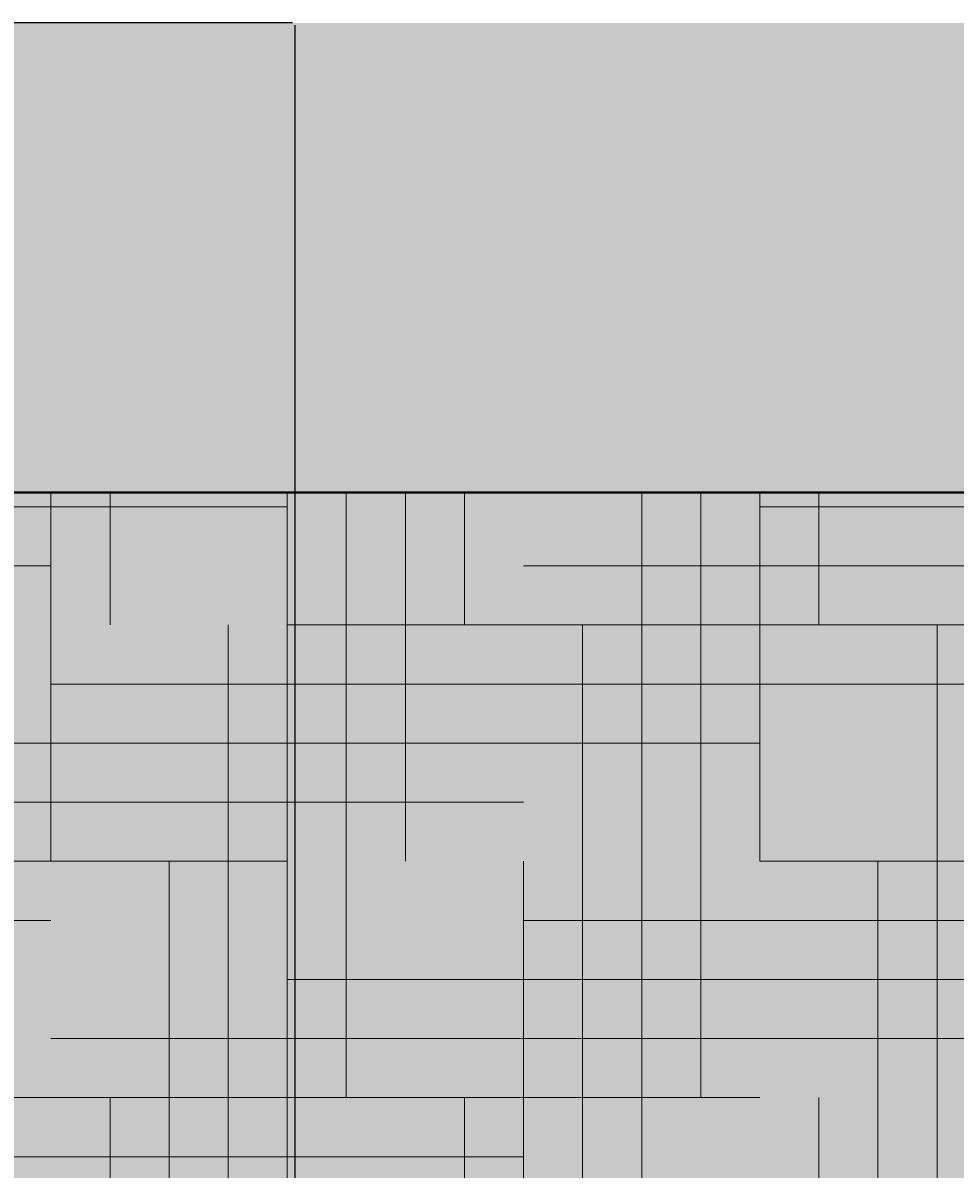
# Model space of a CAD drawing. Units: feet. Extents: x 2695 to 2912, y 795 to 1139.
# Tile 14 of 83: x 2723 to 2748, y 906 to 937. Entities that reach past the tile are written whole.
import ezdxf

# ---------------------------------------------------------------- set-up
doc = ezdxf.new("R2010")
doc.units = ezdxf.units.FT
for name, color, linetype, lineweight in [('A-ANNO-DIMS', 2, 'Continuous', 18), ('A-ELEV', 7, 'Continuous', 35), ('A-ELEV-PATT', 252, 'Continuous', 13)]:
    doc.layers.add(name, color=color, linetype=linetype, lineweight=lineweight)
doc.styles.get("Standard").update_dxf_attribs({"font": 'arial.ttf'})
doc.dimstyles.get("Standard").update_dxf_attribs({"dimtxt": 0.18, "dimasz": 0.18, "dimexe": 0.18, "dimexo": 0.0625, "dimgap": 0.09, "dimtad": 0, "dimtih": 1, "dimtoh": 1, "dimdec": 1, "dimzin": 0, "dimdsep": 46, "dimlunit": 3, "dimtxsty": 'Standard', "dimcen": 0.09, "dimadec": 0, "dimazin": 0, "dimtfac": 1, "dimtdec": 1, "dimtofl": 0, "dimtmove": 0, "dimatfit": 3, "dimfxl": 1, "dimtolj": 1, "dimtzin": 0, "dimarcsym": 0})

# ---------------------------------------------------------------- blocks, each defined once
blk = doc.blocks.new('*D23')
at = {"layer": 'A-ANNO-DIMS', "color": 0, "lineweight": -2, "transparency": 16777216}
for p, q in [((2715.885, 936.868), (2715.885, 794.976)), ((2730.708, 936.868), (2730.708, 794.976)), ((2716.065, 795.156), (2722.842, 795.156)), ((2730.528, 795.156), (2723.752, 795.156))]:
    blk.add_line(p, q, dxfattribs=at)
at = {"layer": 'A-ANNO-DIMS', "color": 0, "transparency": 16777216}
for points in [[(2716.065, 795.186), (2716.065, 795.126), (2715.885, 795.156)], [(2730.528, 795.186), (2730.528, 795.126), (2730.708, 795.156)]]:
    blk.add_solid(points, dxfattribs=at)
at = {"layer": 'Defpoints', "color": 0, "transparency": 16777216}
for p in [(2715.885, 936.931), (2730.708, 936.931), (2730.708, 795.156)]:
    blk.add_point(p, dxfattribs=at)
at = {"layer": 'A-ANNO-DIMS', "color": 0, "transparency": 16777216, "insert": (2723.297, 795.156), "char_height": 0.18, "attachment_point": 5}
blk.add_mtext('\\A1;14.823', dxfattribs=at)
blk = doc.blocks.new('*D24')
at = {"layer": 'A-ANNO-DIMS', "color": 0, "lineweight": -2, "transparency": 16777216}
for p, q in [((2730.708, 936.868), (2730.708, 794.976)), ((2755.112, 936.868), (2755.112, 794.976)), ((2730.888, 795.156), (2742.446, 795.156)), ((2754.932, 795.156), (2743.375, 795.156))]:
    blk.add_line(p, q, dxfattribs=at)
at = {"layer": 'A-ANNO-DIMS', "color": 0, "transparency": 16777216}
for points in [[(2730.888, 795.186), (2730.888, 795.126), (2730.708, 795.156)], [(2754.932, 795.186), (2754.932, 795.126), (2755.112, 795.156)]]:
    blk.add_solid(points, dxfattribs=at)
at = {"layer": 'Defpoints', "color": 0, "transparency": 16777216}
for p in [(2730.708, 936.931), (2755.112, 936.931), (2755.112, 795.156)]:
    blk.add_point(p, dxfattribs=at)
at = {"layer": 'A-ANNO-DIMS', "color": 0, "transparency": 16777216, "insert": (2742.91, 795.156), "char_height": 0.18, "attachment_point": 5}
blk.add_mtext('\\A1;24.404', dxfattribs=at)
blk = doc.blocks.new('*D27')
at = {"layer": 'A-ANNO-DIMS', "color": 0, "lineweight": -2, "transparency": 16777216}
for p, q in [((2730.646, 938.518), (2694.681, 938.518)), ((2694.861, 938.338), (2694.861, 937.906)), ((2694.861, 937.111), (2694.861, 937.542)), ((2730.646, 936.931), (2694.681, 936.931))]:
    blk.add_line(p, q, dxfattribs=at)
at = {"layer": 'A-ANNO-DIMS', "color": 0, "transparency": 16777216}
for points in [[(2694.831, 938.338), (2694.891, 938.338), (2694.861, 938.518)], [(2694.831, 937.111), (2694.891, 937.111), (2694.861, 936.931)]]:
    blk.add_solid(points, dxfattribs=at)
at = {"layer": 'Defpoints', "color": 0, "transparency": 16777216}
for p in [(2694.861, 938.518), (2730.708, 938.518), (2730.708, 936.931)]:
    blk.add_point(p, dxfattribs=at)
at = {"layer": 'A-ANNO-DIMS', "color": 0, "transparency": 16777216, "insert": (2694.861, 937.724), "char_height": 0.18, "attachment_point": 5}
blk.add_mtext('\\A1;1.59', dxfattribs=at)

msp = doc.modelspace()

# ---------------------------------------------------------------- hatches: boundary and pattern name
at = {"layer": 'A-ELEV-PATT'}
h = msp.add_hatch(color=256, dxfattribs=at)
h.set_gradient(color1=(255, 255, 255), tint=1)
h.paths.add_polyline_path([(2770.6361, 1122.9306), (2710.6361, 1122.9306), (2710.6361, 1118.4096), (2770.6361, 1118.4096)])
h.paths.add_polyline_path([(2890.6361, 1107.8588), (2770.6361, 1107.8588), (2770.6361, 1103.3378), (2890.6361, 1103.3378)])
h.paths.add_polyline_path([(2890.6361, 1062.9306), (2710.6361, 1062.9306), (2710.6361, 1056.9306), (2710.6361, 936.9306), (2710.6361, 924.3105), (2716.5358, 924.3105), (2890.6361, 924.3105), (2890.6361, 936.9306), (2715.8852, 936.9306), (2715.8852, 1050.3105), (2890.6361, 1050.3105)])
h.paths.add_polyline_path([(2716.5358, 924.3105), (2710.6361, 924.3105), (2710.6361, 810.9306), (2716.5358, 810.9306)])
h = msp.add_hatch(color=256, dxfattribs=at)
h.set_gradient(color1=(255, 255, 255))
h.paths.add_polyline_path([(2770.6361, 924.3105), (2716.5358, 924.3105), (2716.5358, 810.9306), (2770.6361, 810.9306)])
h.paths.add_polyline_path([(2758.1515, 902.577), (2758.1515, 874.8571), (2724.1893, 874.8571), (2724.1893, 902.577)], flags=16)
h.paths.add_polyline_path([(2756.1515, 900.577), (2756.1515, 876.8571), (2726.1893, 876.8571), (2726.1893, 900.577)], flags=0)
h.paths.add_polyline_path([(2740.7302, 900.577), (2741.6105, 900.577), (2741.6105, 876.8571), (2740.7302, 876.8571)], flags=0)
h = msp.add_hatch(dxfattribs=at)
h.set_pattern_fill('HOUND', color=256, style=0)
h.paths.add_polyline_path([(2770.6361, 924.3105), (2716.5358, 924.3105), (2716.5358, 810.9306), (2770.6361, 810.9306)])
h.paths.add_polyline_path([(2724.1893, 874.8571), (2724.1893, 902.577), (2758.1515, 902.577), (2758.1515, 874.8571)], flags=16)
h.paths.add_polyline_path([(2756.1515, 876.8571), (2726.1893, 876.8571), (2726.1893, 900.577), (2756.1515, 900.577)], flags=0)
h.paths.add_polyline_path([(2741.6105, 876.8571), (2740.7302, 876.8571), (2740.7302, 900.577), (2741.6105, 900.577)], flags=0)

# ---------------------------------------------------------------- linework, layer by layer
at = {"layer": 'A-ELEV'}
msp.add_line((2770.6361, 924.3105), (2716.5358, 924.3105), dxfattribs=at)
msp.add_lwpolyline([(2890.6361, 936.9306), (2890.6361, 924.3105), (2710.6361, 924.3105), (2710.6361, 936.9306)], dxfattribs=at)
msp.add_lwpolyline([(2716.5358, 924.3105), (2770.6361, 924.3105), (2770.6361, 810.9306), (2716.5358, 810.9306)], close=True, dxfattribs=at)

# ---------------------------------------------------------------- dimensions: what is measured, and where the dimension line sits
at = {"layer": 'A-ANNO-DIMS'}
dim = msp.add_linear_dim(base=(2694.8611, 938.5179), p1=(2730.7081, 936.9306), p2=(2730.7081, 938.5179), angle=90, dimstyle='Standard', override={"dimdec": 2, "dimlfac": 1, "dimrnd": 0, "dimzin": 0, "dimdsep": 46, "dimlunit": 2}, dxfattribs=at)
dim.commit()
dim.dimension.update_dxf_attribs({"geometry": '*D27', "text_midpoint": (2694.8611, 937.7242)})
for base, p1, p2, picture, middle in [((2730.7081, 795.1556), (2715.8852, 936.9306), (2730.7081, 936.9306), '*D23', (2723.2967, 795.1556)), ((2755.1125, 795.1556), (2730.7081, 936.9306), (2755.1125, 936.9306), '*D24', (2742.9103, 795.1556))]:
    dim = msp.add_linear_dim(base=base, p1=p1, p2=p2, dimstyle='Standard', override={"dimdec": 3, "dimlfac": 1, "dimrnd": 0, "dimzin": 0, "dimdsep": 46, "dimlunit": 2}, dxfattribs=at)
    dim.commit()
    dim.dimension.update_dxf_attribs({"geometry": picture, "text_midpoint": middle})

doc.saveas('drawing.dxf')
